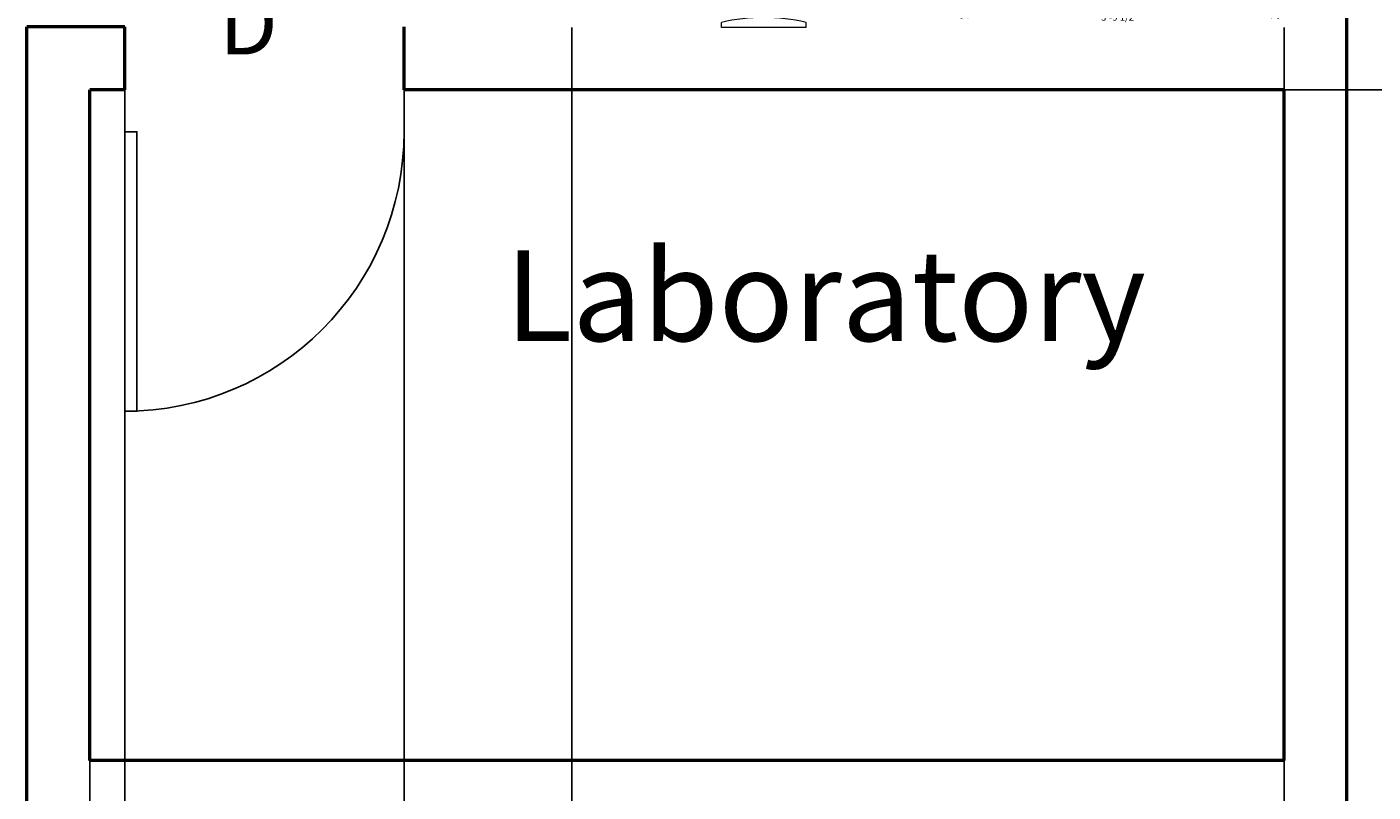
# Model space of a CAD drawing. Units: inches. Extents: x -364 to 705, y -52 to 1250.
# Tile 16 of 34: x 359 to 551, y 308 to 417. Entities that reach past the tile are written whole.
import ezdxf

# ---------------------------------------------------------------- set-up
doc = ezdxf.new("R2010")
doc.units = ezdxf.units.IN
doc.header["$MEASUREMENT"] = 0
for name, color, linetype, lineweight in [('A-ANNO-DIMS', 4, 'Continuous', 18), ('A-ANNO-IDEN', 1, 'Continuous', 18), ('A-AREA-IDEN', 3, 'Continuous', 18), ('A-DOOR', 1, 'Continuous', 25), ('A-FURN', 8, 'Continuous', 18), ('A-WALL', 41, 'Continuous', 50)]:
    doc.layers.add(name, color=color, linetype=linetype, lineweight=lineweight)
doc.styles.get("Standard").update_dxf_attribs({"font": 'arial.ttf'})
doc.dimstyles.get("Standard").update_dxf_attribs({"dimtxt": 1, "dimasz": 1, "dimexe": 0.18, "dimexo": 0.0625, "dimgap": 0.09, "dimtad": 0, "dimtih": 1, "dimtoh": 1, "dimdec": 0, "dimzin": 0, "dimdsep": 46, "dimlunit": 3, "dimtxsty": 'Standard', "dimcen": 0.09, "dimadec": 0, "dimazin": 0, "dimtfac": 1, "dimtdec": 0, "dimtofl": 0, "dimtmove": 0, "dimatfit": 3, "dimfxl": 1, "dimtolj": 1, "dimtzin": 0, "dimarcsym": 0})

# ---------------------------------------------------------------- blocks, each defined once
blk = doc.blocks.new('Chair - Desk')
for p, q in [((-8.5, 0), (-8.5, -1)), ((-8.5, 0), (8.5, 0)), ((8.5, 0), (8.5, -1)), ((-2, -3), (-2, -1.9355)), ((2, -1.9576), (2, -3)), ((-10.5, -5), (-10.5, -14)), ((-8.5, -3), (-8.5, -4)), ((-8.5, -3), (8.5, -3)), ((-6.5, -14), (-6.5, -5)), ((6.5, -5), (6.5, -14)), ((8.5, -3), (8.5, -4)), ((10.5, -14), (10.5, -5)), ((-8.5, -15), (-8.5, -16)), ((8.5, -15), (8.5, -16))]:
    blk.add_line(p, q)
for centre, radius, start, end in [((0, 34.625), 36.625, 256.5803, 283.4197), ((-8.5, -6.5), 2.5, 36.8699, 143.1301), ((8.5, -6.5), 2.5, 36.8699, 143.1301), ((-8.5, -12.5), 2.5, 216.8699, 323.1301), ((0, 19.625), 36.625, 256.5803, 283.4197), ((8.5, -12.5), 2.5, 216.8699, 323.1301)]:
    blk.add_arc(centre, radius, start, end)
blk = doc.blocks.new('*U4')
for p, q in [((0, 0), (0, 6)), ((40, 0), (40, 6))]:
    blk.add_line(p, q)
blk.add_lwpolyline([(0, 0), (0, -40), (1.75, -40), (1.75, 0)], close=True)
blk.add_arc((0, 0), 40, 270, 0)
blk = doc.blocks.new('*D61')
at = {"layer": 'A-ANNO-DIMS', "color": 0, "lineweight": -2, "transparency": 16777216}
for p, q in [((492.39, 427.53), (492.39, 418.34)), ((537.72, 427.53), (537.72, 418.34)), ((493.39, 418.52), (512.47, 418.52)), ((536.72, 418.52), (517.64, 418.52))]:
    blk.add_line(p, q, dxfattribs=at)
at = {"layer": 'A-ANNO-DIMS', "color": 0, "transparency": 16777216}
for points in [[(493.39, 418.69), (493.39, 418.35), (492.39, 418.52)], [(536.72, 418.69), (536.72, 418.35), (537.72, 418.52)]]:
    blk.add_solid(points, dxfattribs=at)
at = {"layer": 'Defpoints', "color": 0, "transparency": 16777216}
for p in [(492.39, 427.59), (537.72, 427.59), (537.72, 418.52)]:
    blk.add_point(p, dxfattribs=at)
at = {"layer": 'A-ANNO-DIMS', "color": 0, "transparency": 16777216, "insert": (515.06, 418.52), "char_height": 1, "attachment_point": 5}
blk.add_mtext('\\A1;3\'-9 1/2"', dxfattribs=at)
blk = doc.blocks.new('*D79')
at = {"layer": 'A-ANNO-DIMS', "color": 0, "lineweight": -2, "transparency": 16777216}
for p, q in [((538.64, 408.11), (703.01, 408.11)), ((702.83, 407.11), (702.83, 356.22)), ((702.83, 304.11), (702.83, 355.01)), ((538.64, 303.11), (703.01, 303.11))]:
    blk.add_line(p, q, dxfattribs=at)
at = {"layer": 'A-ANNO-DIMS', "color": 0, "transparency": 16777216}
for points in [[(702.66, 407.11), (703, 407.11), (702.83, 408.11)], [(702.66, 304.11), (703, 304.11), (702.83, 303.11)]]:
    blk.add_solid(points, dxfattribs=at)
at = {"layer": 'Defpoints', "color": 0, "transparency": 16777216}
for p in [(538.58, 408.11), (702.83, 408.11), (538.58, 303.11)]:
    blk.add_point(p, dxfattribs=at)
at = {"layer": 'A-ANNO-DIMS', "color": 0, "transparency": 16777216, "insert": (702.83, 355.61), "char_height": 1, "attachment_point": 5}
blk.add_mtext('\\A1;8\'-9"', dxfattribs=at)
blk = doc.blocks.new('*D80')
at = {"layer": 'A-ANNO-DIMS', "color": 0, "lineweight": -2, "transparency": 16777216}
for p, q in [((538.64, 531.11), (703.01, 531.11)), ((702.83, 530.11), (702.83, 470.22)), ((702.83, 409.11), (702.83, 469.01)), ((538.64, 408.11), (703.01, 408.11))]:
    blk.add_line(p, q, dxfattribs=at)
at = {"layer": 'A-ANNO-DIMS', "color": 0, "transparency": 16777216}
for points in [[(702.66, 530.11), (703, 530.11), (702.83, 531.11)], [(702.66, 409.11), (703, 409.11), (702.83, 408.11)]]:
    blk.add_solid(points, dxfattribs=at)
at = {"layer": 'Defpoints', "color": 0, "transparency": 16777216}
for p in [(538.58, 531.11), (702.83, 531.11), (538.58, 408.11)]:
    blk.add_point(p, dxfattribs=at)
at = {"layer": 'A-ANNO-DIMS', "color": 0, "transparency": 16777216, "insert": (702.83, 469.61), "char_height": 1, "attachment_point": 5}
blk.add_mtext('\\A1;10\'-3"', dxfattribs=at)
blk = doc.blocks.new('*D100')
at = {"layer": 'A-ANNO-DIMS', "color": 0, "lineweight": -2, "transparency": 16777216}
for p, q in [((436.58, 417.05), (436.58, -51.32)), ((538.58, 417.05), (538.58, -51.32)), ((437.58, -51.14), (486.16, -51.14)), ((537.58, -51.14), (489, -51.14))]:
    blk.add_line(p, q, dxfattribs=at)
at = {"layer": 'A-ANNO-DIMS', "color": 0, "transparency": 16777216}
for points in [[(437.58, -50.97), (437.58, -51.3), (436.58, -51.14)], [(537.58, -50.97), (537.58, -51.3), (538.58, -51.14)]]:
    blk.add_solid(points, dxfattribs=at)
at = {"layer": 'Defpoints', "color": 0, "transparency": 16777216}
for p in [(436.58, 417.11), (538.58, 417.11), (538.58, -51.14)]:
    blk.add_point(p, dxfattribs=at)
at = {"layer": 'A-ANNO-DIMS', "color": 0, "transparency": 16777216, "insert": (487.58, -51.14), "char_height": 1, "attachment_point": 5}
blk.add_mtext('\\A1;8\'-6"', dxfattribs=at)
blk = doc.blocks.new('*D101')
at = {"layer": 'A-ANNO-DIMS', "color": 0, "lineweight": -2, "transparency": 16777216}
for p, q in [((372.58, 408.05), (372.58, -51.32)), ((412.58, 408.05), (412.58, -51.32)), ((373.58, -51.14), (391.16, -51.14)), ((411.58, -51.14), (394, -51.14))]:
    blk.add_line(p, q, dxfattribs=at)
at = {"layer": 'A-ANNO-DIMS', "color": 0, "transparency": 16777216}
for points in [[(373.58, -50.97), (373.58, -51.3), (372.58, -51.14)], [(411.58, -50.97), (411.58, -51.3), (412.58, -51.14)]]:
    blk.add_solid(points, dxfattribs=at)
at = {"layer": 'Defpoints', "color": 0, "transparency": 16777216}
for p in [(372.58, 408.11), (412.58, 408.11), (412.58, -51.14)]:
    blk.add_point(p, dxfattribs=at)
at = {"layer": 'A-ANNO-DIMS', "color": 0, "transparency": 16777216, "insert": (392.58, -51.14), "char_height": 1, "attachment_point": 5}
blk.add_mtext('\\A1;3\'-4"', dxfattribs=at)
blk = doc.blocks.new('*D102')
at = {"layer": 'A-ANNO-DIMS', "color": 0, "lineweight": -2, "transparency": 16777216}
for p, q in [((367.58, 408.05), (367.58, -51.32)), ((372.58, 408.05), (372.58, -51.32)), ((366.58, -51.14), (365.58, -51.14)), ((373.58, -51.14), (374.58, -51.14))]:
    blk.add_line(p, q, dxfattribs=at)
at = {"layer": 'A-ANNO-DIMS', "color": 0, "transparency": 16777216}
for points in [[(366.58, -50.97), (366.58, -51.3), (367.58, -51.14)], [(373.58, -50.97), (373.58, -51.3), (372.58, -51.14)]]:
    blk.add_solid(points, dxfattribs=at)
at = {"layer": 'Defpoints', "color": 0, "transparency": 16777216}
for p in [(367.58, 408.11), (372.58, 408.11), (372.58, -51.14)]:
    blk.add_point(p, dxfattribs=at)
at = {"layer": 'A-ANNO-DIMS', "color": 0, "transparency": 16777216, "insert": (370.08, -51.14), "char_height": 1, "attachment_point": 5}
blk.add_mtext('\\A1;0\'-5"', dxfattribs=at)

msp = doc.modelspace()

# ---------------------------------------------------------------- linework, layer by layer
at = {"layer": 'A-WALL'}
for p, q in [((547.58, 11.11), (547.58, 986.11)), ((372.58, 417.11), (358.58, 417.11)), ((358.58, 303.11), (358.58, 417.11)), ((372.58, 408.11), (372.58, 417.11)), ((412.58, 408.11), (412.58, 417.11)), ((372.58, 408.11), (367.58, 408.11)), ((367.58, 312.11), (367.58, 408.11)), ((538.58, 408.11), (412.58, 408.11)), ((538.58, 312.11), (538.58, 408.11)), ((538.58, 312.11), (367.58, 312.11))]:
    msp.add_line(p, q, dxfattribs=at)

# ---------------------------------------------------------------- block references
at = {"layer": 'A-DOOR'}
msp.add_blockref('*U4', (372.58, 402.11), dxfattribs=at)
at = {"layer": 'A-FURN', "xscale": 0.7131197330740192, "yscale": 0.7131197330740192, "zscale": 0.7131197330740192, "rotation": 180}
msp.add_blockref('Chair - Desk', (464.09, 417.04), dxfattribs=at)

# ---------------------------------------------------------------- texts
at = {"layer": 'A-ANNO-IDEN', "insert": (386.06, 422.17), "char_height": 9, "attachment_point": 1}
msp.add_mtext_dynamic_manual_height_columns('D', width=16.916, gutter_width=1, heights=[0], dxfattribs=at)
at = {"layer": 'A-AREA-IDEN', "insert": (427.05, 385.16), "char_height": 13, "attachment_point": 1}
msp.add_mtext_dynamic_manual_height_columns('Laboratory', width=111.5304, gutter_width=1, heights=[0], dxfattribs=at)

# ---------------------------------------------------------------- dimensions: what is measured, and where the dimension line sits
at = {"layer": 'A-ANNO-DIMS'}
for base, p1, p2, picture, middle in [((702.83, 531.11), (538.58, 408.11), (538.58, 531.11), '*D80', (702.83, 469.61)), ((702.83, 408.11), (538.58, 303.11), (538.58, 408.11), '*D79', (702.83, 355.61))]:
    dim = msp.add_linear_dim(base=base, p1=p1, p2=p2, angle=90, dimstyle='Standard', override={"dimdec": 1, "dimlfac": 1, "dimrnd": 0, "dimzin": 1, "dimdsep": 46, "dimlunit": 4, "dimfrac": 2}, dxfattribs=at)
    dim.commit()
    dim.dimension.update_dxf_attribs({"geometry": picture, "text_midpoint": middle})
for base, p1, p2, picture, middle in [((537.72, 418.52), (492.39, 427.59), (537.72, 427.59), '*D61', (515.06, 418.52)), ((538.58, -51.14), (436.58, 417.11), (538.58, 417.11), '*D100', (487.58, -51.14)), ((372.58, -51.14), (367.58, 408.11), (372.58, 408.11), '*D102', (370.08, -51.14)), ((412.58, -51.14), (372.58, 408.11), (412.58, 408.11), '*D101', (392.58, -51.14))]:
    dim = msp.add_linear_dim(base=base, p1=p1, p2=p2, dimstyle='Standard', override={"dimdec": 1, "dimlfac": 1, "dimrnd": 0, "dimzin": 1, "dimdsep": 46, "dimlunit": 4, "dimfrac": 2}, dxfattribs=at)
    dim.commit()
    dim.dimension.update_dxf_attribs({"geometry": picture, "text_midpoint": middle})

doc.saveas('drawing.dxf')
